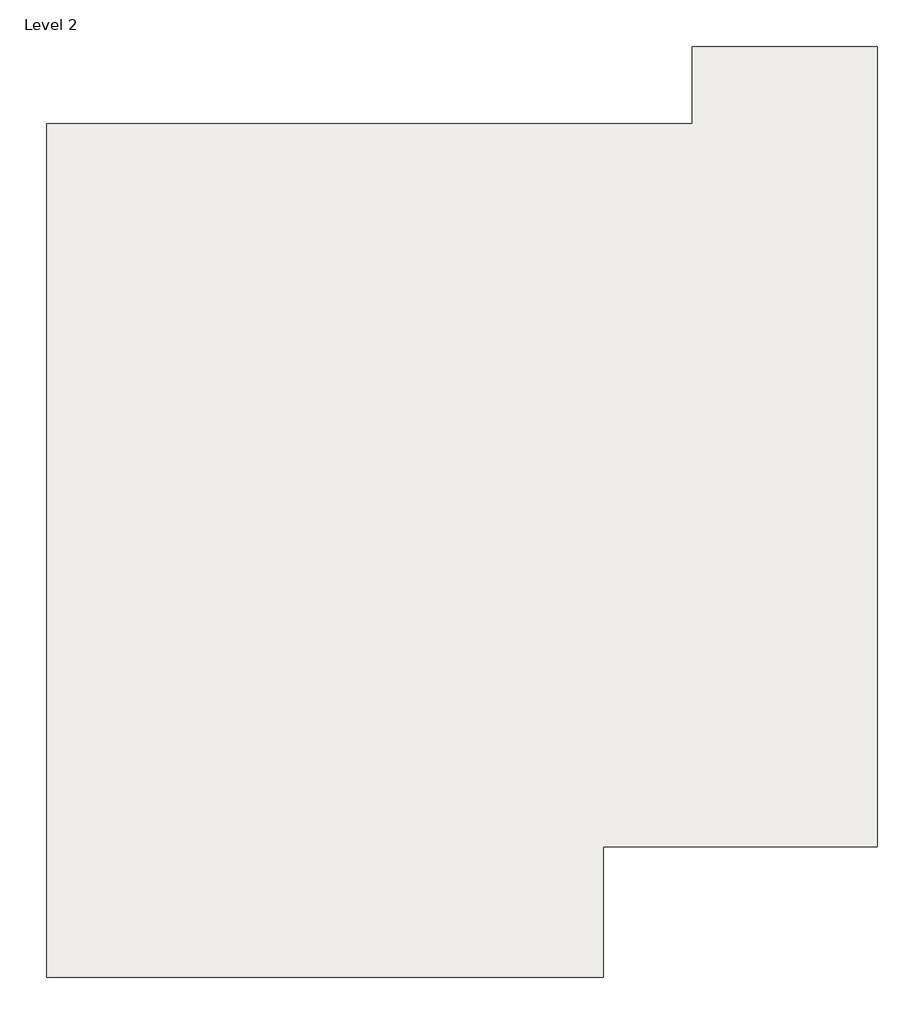
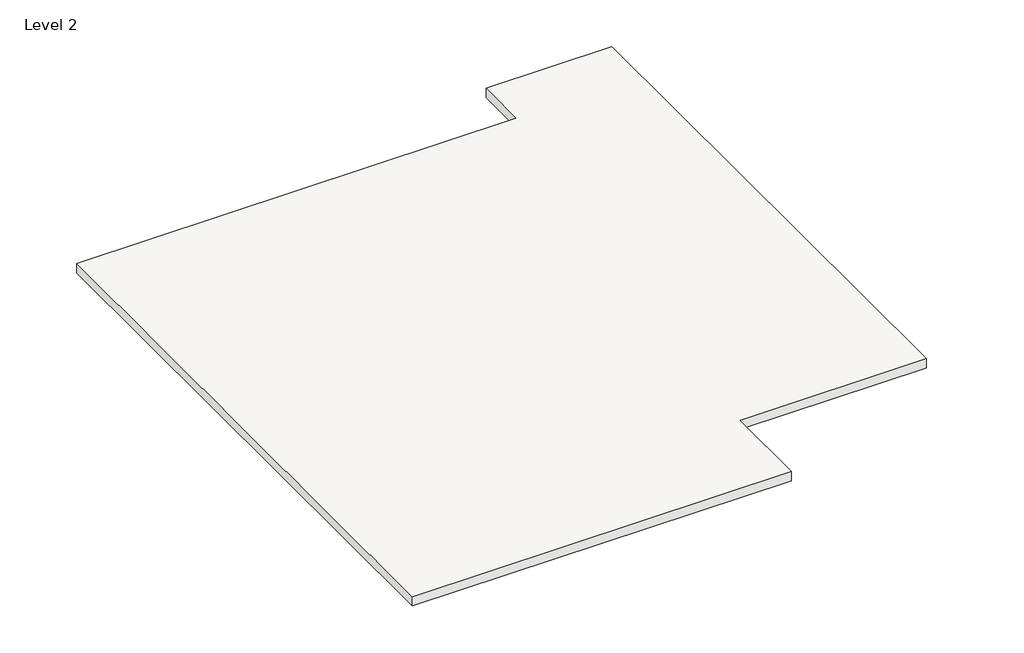
# One storey: 1 roof.
"""IFC4 building model written with IfcOpenShell, lengths in millimetres."""

from ifc_helpers import new_model, si_unit, frame, origin, place, context, project, spatial, polyline, outline, extrude, element, save

model = new_model("IFC4")

# Units and contexts
model_context = context("Model", 3, world=origin())
ifc_project = project(units=[si_unit("LENGTHUNIT", "METRE", prefix="MILLI")], contexts=[model_context])

# Site, building, storey
site = spatial("IfcSite", under=ifc_project)
building = spatial("IfcBuilding", under=site)
storey = spatial("IfcBuildingStorey", under=building, Name="Level 2", Elevation=3048.0)

# Roof
placement = place(None, origin())
element("IfcRoof", 1, ObjectType="Generic - 12\"", at=placement, inside=storey, context=model_context, shape_type="SweptSolid", body=[
    extrude(outline(polyline([(-14211.4918623, 12105.3910469), (-800.2918623, 12105.3910469), (-800.2918623, 13705.5910469), (3035.1081377, 13705.5910469), (3035.1081377, -2906.0089531), (-2654.4918623, -2906.0089531), (-2654.4918623, -5623.8089531), (-14211.4918623, -5623.8089531), (-14211.4918623, 12105.3910469)])), frame((0.0, 0.0, 3048.0), z_axis=(0.0, 0.0, 1.0), x_axis=(1.0, 0.0, 0.0)), (0.0, 0.0, 1.0), 304.8),
])

save(model, "model.ifc")

# Revit data of these elements
# Type "Generic - 12\""
#   Assembly Code = "B1020"
#   Layers, outside or top first: 1' - 0" "Brick, Soldier Course" (function 1)
# Element 1 (IfcRoof, "Generic - 12\"")
#   built-in parameter 1001705 = 11 (stored number, unit not read)
#   built-in parameter 1001710 = 33615
#   Phase Created = New Construction
#   Materials on its faces: "Brick, Soldier Course"
# Materials
#   "Brick, Soldier Course": class "Masonry", colour RGB 170 98 104, transparency 0, Description = "Common brick soldier coursed", Cost = 0
